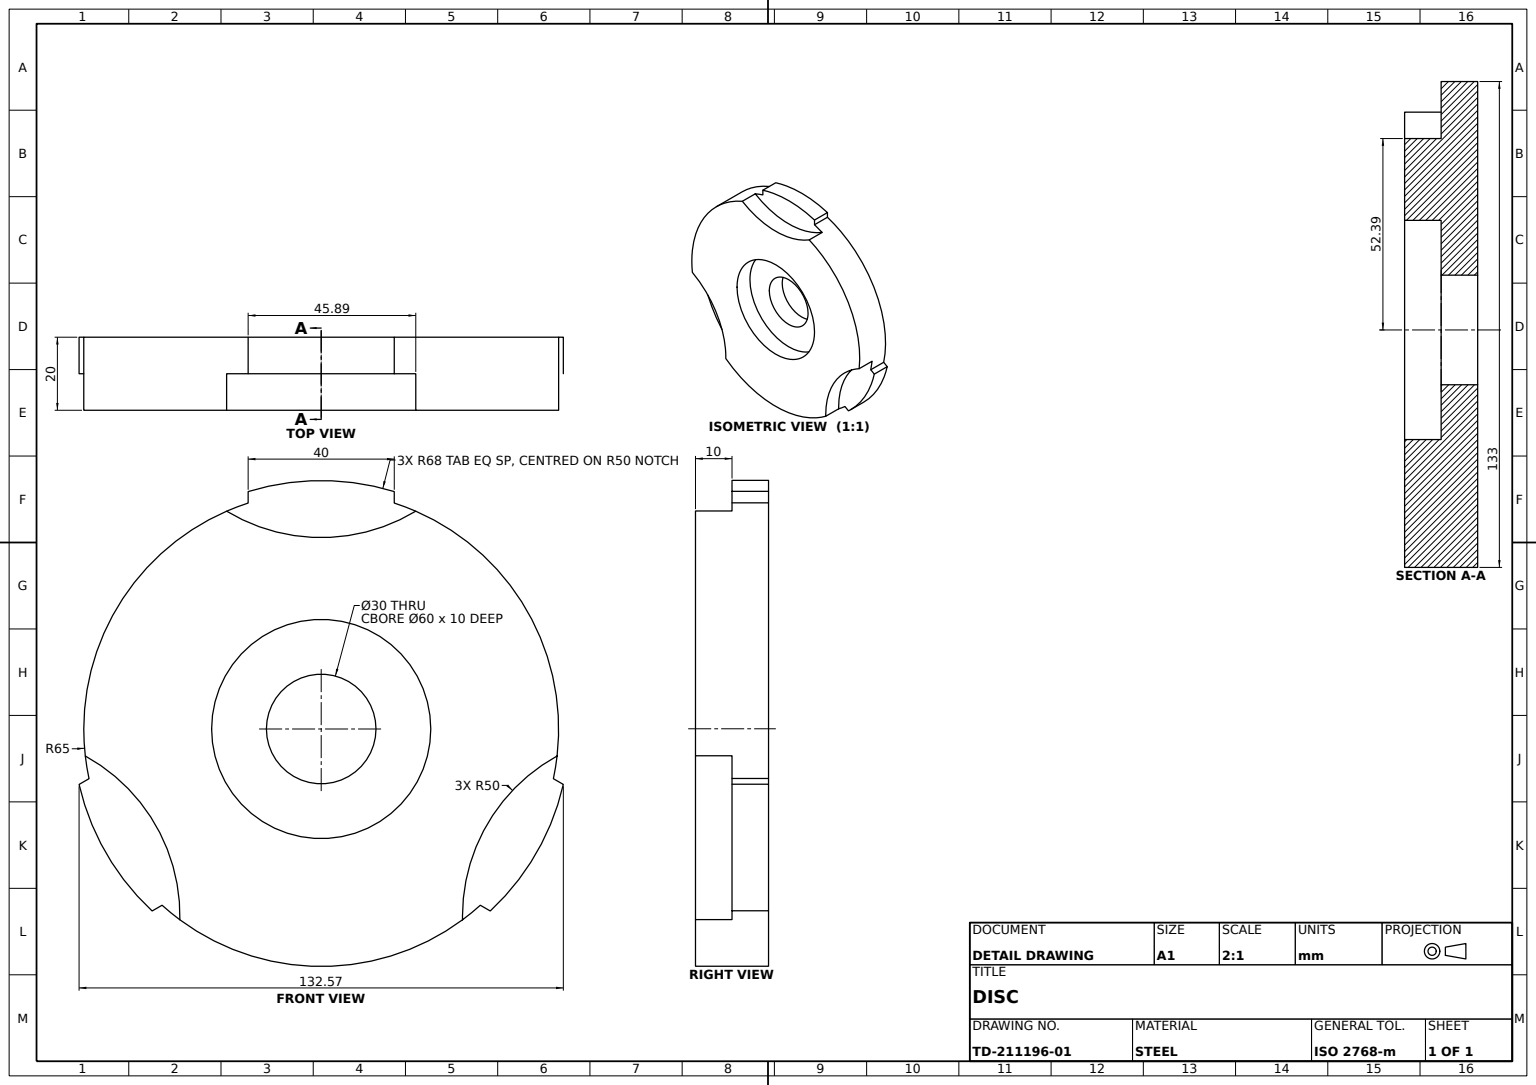
SolidWorks part; units mm, degrees
material "Plain Carbon Steel"
ref_plane "Front Plane" through (0, 0, 0) normal (0, 0, 1) x (1, 0, 0)
ref_plane "Top Plane" through (0, 0, 0) normal (0, 1, 0) x (1, 0, 0)
ref_plane "Right Plane" through (0, 0, 0) normal (1, 0, 0) x (0, 0, -1)
sketch "Base Disc Profile Sketch" plane through (0, 0, 0) normal (0, 0, 1) x (1, 0, 0)
  line L0 (0, 0) -> (82.7041, 0) construction
  line L1 (20, 61.8466) -> (20, 64.9923)
  line L2 (-20, 61.8466) -> (-20, 64.9923)
  line L3 (63.5607, -13.6028) -> (66.285, -15.1756)
  line L4 (43.5607, -48.2438) -> (46.285, -49.8167)
  line L5 (-43.5607, -48.2438) -> (-46.285, -49.8167)
  line L6 (-63.5607, -13.6028) -> (-66.285, -15.1756)
  line L7 (-20, 56.5685) -> (-20, 61.8466) construction
  line L8 (20, 56.5685) -> (20, 61.8466) construction
  line L9 (-38.9898, -45.6048) -> (-43.5607, -48.2438) construction
  line L10 (-58.9898, -10.9638) -> (-63.5607, -13.6028) construction
  line L11 (38.9898, -45.6048) -> (43.5607, -48.2438) construction
  line L12 (58.9898, -10.9638) -> (63.5607, -13.6028) construction
  arc A0 (20, 64.9923) -> (-20, 64.9923) centre (0, 0) ccw
  arc A2 (-20, 61.8466) -> (-63.5607, -13.6028) centre (0, 0) ccw
  arc A3 (20, 61.8466) -> (-20, 61.8466) centre (0, 0) ccw construction
  arc A4 (20, 56.5685) -> (0, 60) centre (0, 0) ccw construction
  arc A5 (46.285, -49.8167) -> (66.285, -15.1756) centre (0, 0) ccw
  arc A6 (-66.285, -15.1756) -> (-46.285, -49.8167) centre (0, 0) ccw
  arc A7 (-38.9898, -45.6048) -> (38.9898, -45.6048) centre (0, 0) ccw construction
  arc A8 (-58.9898, -10.9638) -> (-38.9898, -45.6048) centre (0, 0) ccw construction
  arc A9 (58.9898, -10.9638) -> (60, 0) centre (0, 0) ccw construction
  arc A10 (38.9898, -45.6048) -> (58.9898, -10.9638) centre (0, 0) ccw construction
  arc A11 (60, 0) -> (20, 56.5685) centre (0, 0) ccw construction
  arc A12 (-43.5607, -48.2438) -> (43.5607, -48.2438) centre (0, 0) ccw
  arc A13 (-63.5607, -13.6028) -> (-43.5607, -48.2438) centre (0, 0) ccw construction
  arc A14 (63.5607, -13.6028) -> (20, 61.8466) centre (0, 0) ccw
  arc A15 (43.5607, -48.2438) -> (63.5607, -13.6028) centre (0, 0) ccw construction
  point P3 (20, 0)
  point P5 (20, 107.2704)
  point P6 (-20, 0)
  point P7 (-20, 107.2704)
  point P22 (0, 0)
  dimension "D1" = 3
  dimension "D3" = 65
  dimension "D2" = 68
  dimension "D4" = 60
  dimension "D5" = 40
extrude "Base Disc" add sketch "Base Disc Profile Sketch" along normal blind 10
sketch "Upper Section Sketch" plane through (0, 0, 10) normal (0, 0, 1) x (1, 0, 0)
  line L0 (0, 0) -> (0, 95.1412) construction
  line L1 (-20, 64.9923) -> (-20, 61.8466) construction
  arc A0 (-25.8921, 59.6205) -> (-64.5789, -7.387) centre (0, 0) ccw
  arc A2 (-25.8921, 59.6205) -> (25.8921, 59.6205) centre (0, 102.3943) ccw
  arc A5 (64.5789, -7.387) -> (38.6868, -52.2334) centre (88.6761, -51.1971) ccw
  arc A6 (-38.6868, -52.2334) -> (-64.5789, -7.387) centre (-88.6761, -51.1971) ccw
  arc A7 (-38.6868, -52.2334) -> (38.6868, -52.2334) centre (0, 0) ccw
  arc A9 (64.5789, -7.387) -> (25.8921, 59.6205) centre (0, 0) ccw
  point P15 (0, 0)
  dimension "D1" = 3
  dimension "D2" = 65
  dimension "D3" = 50
  dimension "D4" = 45.8921
extrude "Upper Section" add sketch "Upper Section Sketch" along normal blind 10
sketch "Counterbore Sketch" plane through (0, 0, 20) normal (0, 0, 1) x (1, 0, 0)
  circle A0 centre (0, 0) radius 30
  dimension "D1" = 60
extrude "Counterbore" cut sketch "Counterbore Sketch" against normal blind 10
sketch "Through Bore Sketch" plane through (0, 0, 10) normal (0, 0, 1) x (1, 0, 0)
  circle A0 centre (0, 0) radius 15
  dimension "D1" = 30
extrude "Through Bore" cut sketch "Through Bore Sketch" against normal blind 10
